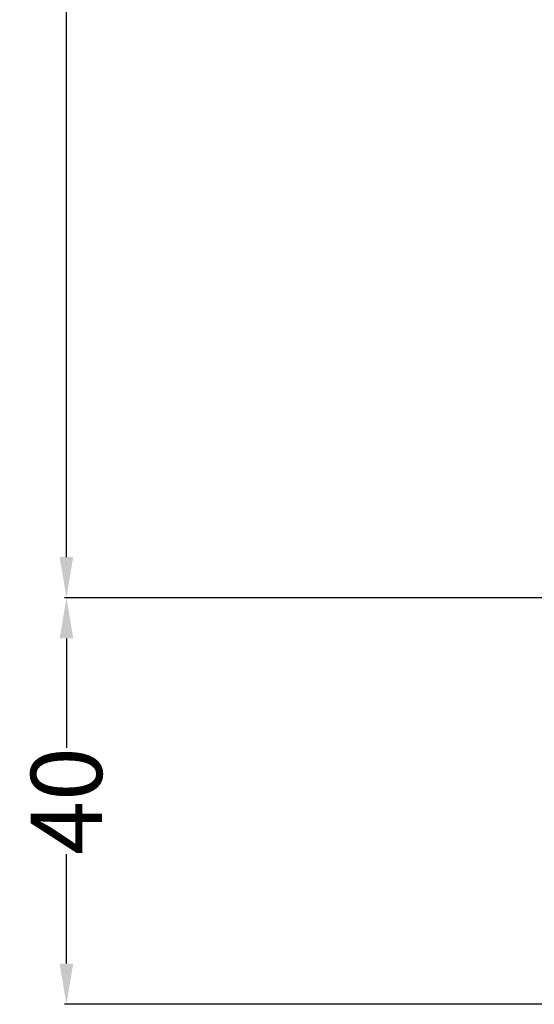
# Model space of a CAD drawing. Units: millimetres. Extents: x 0 to 2267, y 0 to 1823.
# Tile 2 of 256: x 1327 to 1378, y 1077 to 1174. Entities that reach past the tile are written whole.
import ezdxf

# ---------------------------------------------------------------- set-up
doc = ezdxf.new("R2010")
doc.units = ezdxf.units.MM
doc.header["$MEASUREMENT"] = 0
doc.layers.add('M-DIMS', color=2, linetype='Continuous', lineweight=25)
doc.styles.get("Standard").update_dxf_attribs({"font": 'arial.ttf'})
doc.dimstyles.get("Standard").update_dxf_attribs({"dimtxt": 7, "dimasz": 4, "dimexe": 0.18, "dimexo": 0.0625, "dimgap": 0.09, "dimtad": 0, "dimdec": 0, "dimzin": 0, "dimdsep": 46, "dimtxsty": 'Standard', "dimcen": 0.09, "dimadec": 0, "dimazin": 0, "dimtfac": 1, "dimtdec": 0, "dimtofl": 0, "dimtmove": 0, "dimatfit": 3, "dimfxl": 1, "dimtolj": 1, "dimtzin": 0, "dimarcsym": 0})

# ---------------------------------------------------------------- blocks, each defined once
blk = doc.blocks.new('*D9')
at = {"layer": 'Defpoints', "color": 0, "transparency": 16777216}
for p in [(1332.087, 1117.417), (1505.929, 1117.417), (1505.929, 1077.417)]:
    blk.add_point(p, dxfattribs=at)
at = {"layer": 'M-DIMS', "color": 0, "lineweight": -2, "transparency": 16777216}
for p, q in [((1505.866, 1117.417), (1331.907, 1117.417)), ((1332.087, 1113.417), (1332.087, 1102.65)), ((1332.087, 1081.417), (1332.087, 1092.184)), ((1505.866, 1077.417), (1331.907, 1077.417))]:
    blk.add_line(p, q, dxfattribs=at)
at = {"layer": 'M-DIMS', "color": 0, "transparency": 16777216}
for points in [[(1331.42, 1113.417), (1332.753, 1113.417), (1332.087, 1117.417)], [(1331.42, 1081.417), (1332.753, 1081.417), (1332.087, 1077.417)]]:
    blk.add_solid(points, dxfattribs=at)
at = {"layer": 'M-DIMS', "color": 0, "transparency": 16777216, "insert": (1332.087, 1097.417), "char_height": 7, "attachment_point": 5, "rotation": 90}
blk.add_mtext('\\A1;40', dxfattribs=at)
blk = doc.blocks.new('*D10')
at = {"layer": 'Defpoints', "color": 0, "transparency": 16777216}
for p in [(1332.087, 1287.766), (1505.929, 1287.766), (1505.929, 1117.417)]:
    blk.add_point(p, dxfattribs=at)
at = {"layer": 'M-DIMS', "color": 0, "lineweight": -2, "transparency": 16777216}
for p, q in [((1505.866, 1287.766), (1331.907, 1287.766)), ((1332.087, 1283.766), (1332.087, 1216.908)), ((1332.087, 1121.417), (1332.087, 1188.275)), ((1505.866, 1117.417), (1331.907, 1117.417))]:
    blk.add_line(p, q, dxfattribs=at)
at = {"layer": 'M-DIMS', "color": 0, "transparency": 16777216}
for points in [[(1331.42, 1283.766), (1332.753, 1283.766), (1332.087, 1287.766)], [(1331.42, 1121.417), (1332.753, 1121.417), (1332.087, 1117.417)]]:
    blk.add_solid(points, dxfattribs=at)
at = {"layer": 'M-DIMS', "color": 0, "transparency": 16777216, "insert": (1332.087, 1202.591), "char_height": 7, "attachment_point": 5, "rotation": 90}
blk.add_mtext('\\A1;170.35', dxfattribs=at)

msp = doc.modelspace()

# ---------------------------------------------------------------- dimensions: what is measured, and where the dimension line sits
at = {"layer": 'M-DIMS'}
for base, p1, p2, override, picture, middle in [((1332.087, 1287.766), (1505.929, 1117.417), (1505.929, 1287.766), {"dimdec": 2, "dimlfac": 1, "dimrnd": 0, "dimzin": 0, "dimdsep": 46, "dimlunit": 2}, '*D10', (1332.087, 1202.591)), ((1332.087, 1117.417), (1505.929, 1077.417), (1505.929, 1117.417), {"dimdec": 0, "dimlfac": 1, "dimrnd": 0, "dimzin": 0, "dimdsep": 46, "dimlunit": 2}, '*D9', (1332.087, 1097.417))]:
    dim = msp.add_linear_dim(base=base, p1=p1, p2=p2, angle=90, dimstyle='Standard', override=override, dxfattribs=at)
    dim.commit()
    dim.dimension.update_dxf_attribs({"geometry": picture, "text_midpoint": middle})

doc.saveas('drawing.dxf')
